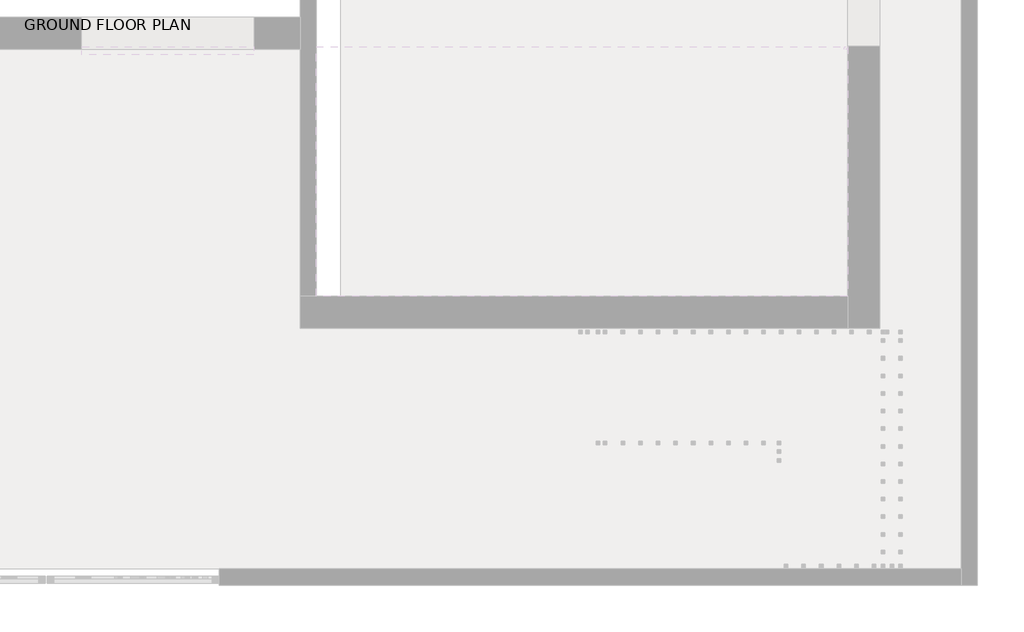
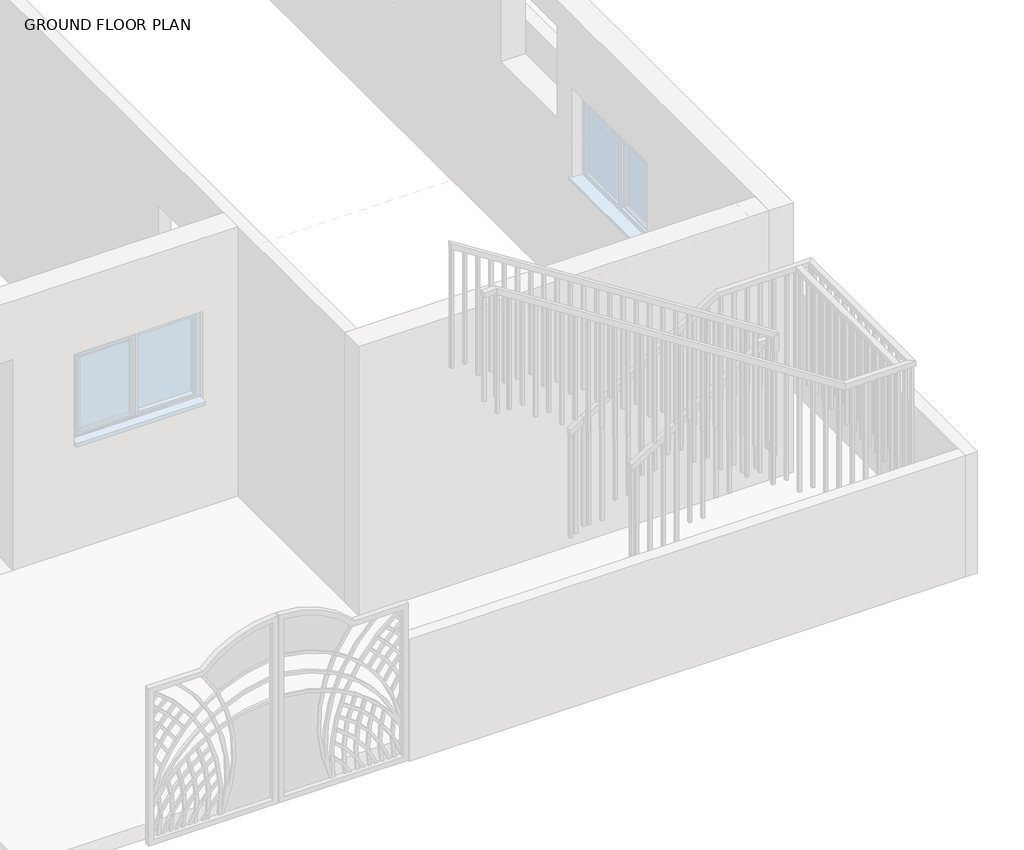
# One storey, part 11 of 23: 2 railings.
"""IFC4 building model written with IfcOpenShell, lengths in millimetres."""

from ifc_helpers import new_model, si_unit, frame, origin, place, context, project, spatial, polyline, outline, extrude, faceted_brep, element, save

model = new_model("IFC4")

# Units and contexts
model_context = context("Model", 3, world=origin())
ifc_project = project(units=[si_unit("LENGTHUNIT", "METRE", prefix="MILLI")], contexts=[model_context])

# Site, building, storey
site = spatial("IfcSite", under=ifc_project)
building = spatial("IfcBuilding", under=site)
storey = spatial("IfcBuildingStorey", under=building, Name="GROUND FLOOR PLAN", Elevation=487.68)

# Railings
placement = place(None, origin())
element("IfcRailing", 1, ObjectType="1100mm", at=placement, inside=storey, context=model_context, shape_type="SolidModel", body=[
    faceted_brep([(-8680.149573, -10220.0521308, 1912.8), (-8680.149573, -10220.0521308, 1853.4423995), (-8680.149573, -10270.0521308, 1853.4423995), (-8680.149573, -10270.0521308, 1912.8), (-7409.7306254, -10220.0521308, 2725.6), (-7395.1045513, -10220.0521308, 2675.6), (-7395.1045513, -10270.0521308, 2675.6), (-7409.7306254, -10270.0521308, 2725.6), (-6495.8132565, -10220.0521308, 2725.6), (-6495.8132565, -10220.0521308, 2675.6), (-6545.8132565, -10270.0521308, 2675.6), (-6545.8132565, -10270.0521308, 2725.6), (-6495.8132565, -11933.6860066, 2725.6), (-6495.8132565, -11933.6860066, 2675.6), (-6545.8132565, -11883.6860066, 2675.6), (-6545.8132565, -11883.6860066, 2725.6), (-7155.718398, -11933.6860066, 2725.6), (-7170.3479429, -11933.6860066, 2675.6), (-7170.3479429, -11883.6860066, 2675.6), (-7155.718398, -11883.6860066, 2725.6), (-10457.8773536, -11933.6860066, 4838.88), (-10457.8773536, -11883.6860066, 4838.88), (-10457.8773536, -11883.6860066, 4779.517542), (-10457.8773536, -11933.6860066, 4779.517542)], [[[0, 1, 2, 3]], [[1, 0, 4, 5]], [[2, 1, 5, 6]], [[3, 2, 6, 7]], [[0, 3, 7, 4]], [[5, 4, 8, 9]], [[6, 5, 9, 10]], [[7, 6, 10, 11]], [[4, 7, 11, 8]], [[9, 8, 12, 13]], [[10, 9, 13, 14]], [[11, 10, 14, 15]], [[8, 11, 15, 12]], [[13, 12, 16, 17]], [[14, 13, 17, 18]], [[15, 14, 18, 19]], [[12, 15, 19, 16]], [[20, 21, 22, 23]], [[17, 16, 20, 23]], [[18, 17, 23, 22]], [[19, 18, 22, 21]], [[16, 19, 21, 20]]]),
    extrude(outline(polyline([(4691.8007425, -10320.8132565), (4707.7999723, -10345.8132565), (3576.32, -10345.8132565), (3576.32, -10320.8132565), (4691.8007425, -10320.8132565)])), frame((0.0, -11921.1860066, 0.0), z_axis=(0.0, 1.0, 0.0), x_axis=(0.0, 0.0, 1.0)), (0.0, 0.0, 1.0), 25.0),
    extrude(outline(polyline([(4611.8045935, -10195.8132565), (4627.8038233, -10220.8132565), (3576.32, -10220.8132565), (3576.32, -10195.8132565), (4611.8045935, -10195.8132565)])), frame((0.0, -11921.1860066, 0.0), z_axis=(0.0, 1.0, 0.0), x_axis=(0.0, 0.0, 1.0)), (0.0, 0.0, 1.0), 25.0),
    extrude(outline(polyline([(4531.8084444, -10070.8132565), (4547.8076742, -10095.8132565), (3413.76, -10095.8132565), (3413.76, -10070.8132565), (4531.8084444, -10070.8132565)])), frame((0.0, -11921.1860066, 0.0), z_axis=(0.0, 1.0, 0.0), x_axis=(0.0, 0.0, 1.0)), (0.0, 0.0, 1.0), 25.0),
    extrude(outline(polyline([(4451.8122954, -9945.8132565), (4467.8115252, -9970.8132565), (3413.76, -9970.8132565), (3413.76, -9945.8132565), (4451.8122954, -9945.8132565)])), frame((0.0, -11921.1860066, 0.0), z_axis=(0.0, 1.0, 0.0), x_axis=(0.0, 0.0, 1.0)), (0.0, 0.0, 1.0), 25.0),
    extrude(outline(polyline([(4371.8161463, -9820.8132565), (4387.8153761, -9845.8132565), (3251.2, -9845.8132565), (3251.2, -9820.8132565), (4371.8161463, -9820.8132565)])), frame((0.0, -11921.1860066, 0.0), z_axis=(0.0, 1.0, 0.0), x_axis=(0.0, 0.0, 1.0)), (0.0, 0.0, 1.0), 25.0),
    extrude(outline(polyline([(4291.8423995, -9695.8132565), (4307.8371231, -9720.8132565), (3251.2, -9720.8132565), (3251.2, -9695.8132565), (4291.8423995, -9695.8132565)])), frame((0.0, -11921.1860066, 0.0), z_axis=(0.0, 1.0, 0.0), x_axis=(0.0, 0.0, 1.0)), (0.0, 0.0, 1.0), 25.0),
    extrude(outline(polyline([(4211.8238482, -9570.8132565), (4227.823078, -9595.8132565), (3088.64, -9595.8132565), (3088.64, -9570.8132565), (4211.8238482, -9570.8132565)])), frame((0.0, -11921.1860066, 0.0), z_axis=(0.0, 1.0, 0.0), x_axis=(0.0, 0.0, 1.0)), (0.0, 0.0, 1.0), 25.0),
    extrude(outline(polyline([(4131.8276992, -9445.8132565), (4147.826929, -9470.8132565), (3088.64, -9470.8132565), (3088.64, -9445.8132565), (4131.8276992, -9445.8132565)])), frame((0.0, -11921.1860066, 0.0), z_axis=(0.0, 1.0, 0.0), x_axis=(0.0, 0.0, 1.0)), (0.0, 0.0, 1.0), 25.0),
    extrude(outline(polyline([(4051.8315501, -9320.8132565), (4067.8307799, -9345.8132565), (2926.08, -9345.8132565), (2926.08, -9320.8132565), (4051.8315501, -9320.8132565)])), frame((0.0, -11921.1860066, 0.0), z_axis=(0.0, 1.0, 0.0), x_axis=(0.0, 0.0, 1.0)), (0.0, 0.0, 1.0), 25.0),
    extrude(outline(polyline([(3971.835401, -9195.8132565), (3987.8346309, -9220.8132565), (2926.08, -9220.8132565), (2926.08, -9195.8132565), (3971.835401, -9195.8132565)])), frame((0.0, -11921.1860066, 0.0), z_axis=(0.0, 1.0, 0.0), x_axis=(0.0, 0.0, 1.0)), (0.0, 0.0, 1.0), 25.0),
    extrude(outline(polyline([(3891.839252, -9070.8132565), (3907.8384818, -9095.8132565), (2763.52, -9095.8132565), (2763.52, -9070.8132565), (3891.839252, -9070.8132565)])), frame((0.0, -11921.1860066, 0.0), z_axis=(0.0, 1.0, 0.0), x_axis=(0.0, 0.0, 1.0)), (0.0, 0.0, 1.0), 25.0),
    extrude(outline(polyline([(3811.8431029, -8945.8132565), (3827.8423328, -8970.8132565), (2763.52, -8970.8132565), (2763.52, -8945.8132565), (3811.8431029, -8945.8132565)])), frame((0.0, -11921.1860066, 0.0), z_axis=(0.0, 1.0, 0.0), x_axis=(0.0, 0.0, 1.0)), (0.0, 0.0, 1.0), 25.0),
    extrude(outline(polyline([(3731.8469539, -8820.8132565), (3747.8461837, -8845.8132565), (2600.96, -8845.8132565), (2600.96, -8820.8132565), (3731.8469539, -8820.8132565)])), frame((0.0, -11921.1860066, 0.0), z_axis=(0.0, 1.0, 0.0), x_axis=(0.0, 0.0, 1.0)), (0.0, 0.0, 1.0), 25.0),
    extrude(outline(polyline([(3651.8508048, -8695.8132565), (3667.8500347, -8720.8132565), (2600.96, -8720.8132565), (2600.96, -8695.8132565), (3651.8508048, -8695.8132565)])), frame((0.0, -11921.1860066, 0.0), z_axis=(0.0, 1.0, 0.0), x_axis=(0.0, 0.0, 1.0)), (0.0, 0.0, 1.0), 25.0),
    extrude(outline(polyline([(3571.8546558, -8570.8132565), (3587.8538856, -8595.8132565), (2438.4, -8595.8132565), (2438.4, -8570.8132565), (3571.8546558, -8570.8132565)])), frame((0.0, -11921.1860066, 0.0), z_axis=(0.0, 1.0, 0.0), x_axis=(0.0, 0.0, 1.0)), (0.0, 0.0, 1.0), 25.0),
    extrude(outline(polyline([(3491.8585067, -8445.8132565), (3507.8577365, -8470.8132565), (2438.4, -8470.8132565), (2438.4, -8445.8132565), (3491.8585067, -8445.8132565)])), frame((0.0, -11921.1860066, 0.0), z_axis=(0.0, 1.0, 0.0), x_axis=(0.0, 0.0, 1.0)), (0.0, 0.0, 1.0), 25.0),
    extrude(outline(polyline([(3411.8623577, -8320.8132565), (3427.8615875, -8345.8132565), (2275.84, -8345.8132565), (2275.84, -8320.8132565), (3411.8623577, -8320.8132565)])), frame((0.0, -11921.1860066, 0.0), z_axis=(0.0, 1.0, 0.0), x_axis=(0.0, 0.0, 1.0)), (0.0, 0.0, 1.0), 25.0),
    extrude(outline(polyline([(3331.8662086, -8195.8132565), (3347.8654384, -8220.8132565), (2275.84, -8220.8132565), (2275.84, -8195.8132565), (3331.8662086, -8195.8132565)])), frame((0.0, -11921.1860066, 0.0), z_axis=(0.0, 1.0, 0.0), x_axis=(0.0, 0.0, 1.0)), (0.0, 0.0, 1.0), 25.0),
    extrude(outline(polyline([(3251.8700596, -8070.8132565), (3267.8692894, -8095.8132565), (2113.28, -8095.8132565), (2113.28, -8070.8132565), (3251.8700596, -8070.8132565)])), frame((0.0, -11921.1860066, 0.0), z_axis=(0.0, 1.0, 0.0), x_axis=(0.0, 0.0, 1.0)), (0.0, 0.0, 1.0), 25.0),
    extrude(outline(polyline([(3171.8739105, -7945.8132565), (3187.8731403, -7970.8132565), (2113.28, -7970.8132565), (2113.28, -7945.8132565), (3171.8739105, -7945.8132565)])), frame((0.0, -11921.1860066, 0.0), z_axis=(0.0, 1.0, 0.0), x_axis=(0.0, 0.0, 1.0)), (0.0, 0.0, 1.0), 25.0),
    extrude(outline(polyline([(3091.8777615, -7820.8132565), (3107.8769913, -7845.8132565), (1950.72, -7845.8132565), (1950.72, -7820.8132565), (3091.8777615, -7820.8132565)])), frame((0.0, -11921.1860066, 0.0), z_axis=(0.0, 1.0, 0.0), x_axis=(0.0, 0.0, 1.0)), (0.0, 0.0, 1.0), 25.0),
    extrude(outline(polyline([(3011.8816124, -7695.8132565), (3027.8808422, -7720.8132565), (1950.72, -7720.8132565), (1950.72, -7695.8132565), (3011.8816124, -7695.8132565)])), frame((0.0, -11921.1860066, 0.0), z_axis=(0.0, 1.0, 0.0), x_axis=(0.0, 0.0, 1.0)), (0.0, 0.0, 1.0), 25.0),
    extrude(outline(polyline([(2931.8854634, -7570.8132565), (2947.8846932, -7595.8132565), (1788.16, -7595.8132565), (1788.16, -7570.8132565), (2931.8854634, -7570.8132565)])), frame((0.0, -11921.1860066, 0.0), z_axis=(0.0, 1.0, 0.0), x_axis=(0.0, 0.0, 1.0)), (0.0, 0.0, 1.0), 25.0),
    extrude(outline(polyline([(2851.8893143, -7445.8132565), (2867.8885441, -7470.8132565), (1788.16, -7470.8132565), (1788.16, -7445.8132565), (2851.8893143, -7445.8132565)])), frame((0.0, -11921.1860066, 0.0), z_axis=(0.0, 1.0, 0.0), x_axis=(0.0, 0.0, 1.0)), (0.0, 0.0, 1.0), 25.0),
    extrude(outline(polyline([(2771.8931653, -7320.8132565), (2787.8923951, -7345.8132565), (1625.6, -7345.8132565), (1625.6, -7320.8132565), (2771.8931653, -7320.8132565)])), frame((0.0, -11921.1860066, 0.0), z_axis=(0.0, 1.0, 0.0), x_axis=(0.0, 0.0, 1.0)), (0.0, 0.0, 1.0), 25.0),
    extrude(outline(polyline([(2691.8970162, -7195.8132565), (2707.896246, -7220.8132565), (1625.6, -7220.8132565), (1625.6, -7195.8132565), (2691.8970162, -7195.8132565)])), frame((0.0, -11921.1860066, 0.0), z_axis=(0.0, 1.0, 0.0), x_axis=(0.0, 0.0, 1.0)), (0.0, 0.0, 1.0), 25.0),
    extrude(outline(polyline([(-7070.8132565, -11921.1860066), (-7095.8132565, -11921.1860066), (-7095.8132565, -11896.1860066), (-7070.8132565, -11896.1860066), (-7070.8132565, -11921.1860066)])), frame((0.0, 0.0, 1625.6), z_axis=(0.0, 0.0, 1.0), x_axis=(1.0, 0.0, 0.0)), (0.0, 0.0, 1.0), 1050.0),
    extrude(outline(polyline([(-6945.8132565, -11921.1860066), (-6970.8132565, -11921.1860066), (-6970.8132565, -11896.1860066), (-6945.8132565, -11896.1860066), (-6945.8132565, -11921.1860066)])), frame((0.0, 0.0, 1625.6), z_axis=(0.0, 0.0, 1.0), x_axis=(1.0, 0.0, 0.0)), (0.0, 0.0, 1.0), 1050.0),
    extrude(outline(polyline([(-6820.8132565, -11921.1860066), (-6845.8132565, -11921.1860066), (-6845.8132565, -11896.1860066), (-6820.8132565, -11896.1860066), (-6820.8132565, -11921.1860066)])), frame((0.0, 0.0, 1625.6), z_axis=(0.0, 0.0, 1.0), x_axis=(1.0, 0.0, 0.0)), (0.0, 0.0, 1.0), 1050.0),
    extrude(outline(polyline([(-6695.8132565, -11921.1860066), (-6720.8132565, -11921.1860066), (-6720.8132565, -11896.1860066), (-6695.8132565, -11896.1860066), (-6695.8132565, -11921.1860066)])), frame((0.0, 0.0, 1625.6), z_axis=(0.0, 0.0, 1.0), x_axis=(1.0, 0.0, 0.0)), (0.0, 0.0, 1.0), 1050.0),
    extrude(outline(polyline([(-6570.8132565, -11921.1860066), (-6595.8132565, -11921.1860066), (-6595.8132565, -11896.1860066), (-6570.8132565, -11896.1860066), (-6570.8132565, -11921.1860066)])), frame((0.0, 0.0, 1625.6), z_axis=(0.0, 0.0, 1.0), x_axis=(1.0, 0.0, 0.0)), (0.0, 0.0, 1.0), 1050.0),
    extrude(outline(polyline([(-6508.3132565, -11795.0521308), (-6508.3132565, -11820.0521308), (-6533.3132565, -11820.0521308), (-6533.3132565, -11795.0521308), (-6508.3132565, -11795.0521308)])), frame((0.0, 0.0, 1625.6), z_axis=(0.0, 0.0, 1.0), x_axis=(1.0, 0.0, 0.0)), (0.0, 0.0, 1.0), 1050.0),
    extrude(outline(polyline([(-6508.3132565, -11670.0521308), (-6508.3132565, -11695.0521308), (-6533.3132565, -11695.0521308), (-6533.3132565, -11670.0521308), (-6508.3132565, -11670.0521308)])), frame((0.0, 0.0, 1625.6), z_axis=(0.0, 0.0, 1.0), x_axis=(1.0, 0.0, 0.0)), (0.0, 0.0, 1.0), 1050.0),
    extrude(outline(polyline([(-6508.3132565, -11545.0521308), (-6508.3132565, -11570.0521308), (-6533.3132565, -11570.0521308), (-6533.3132565, -11545.0521308), (-6508.3132565, -11545.0521308)])), frame((0.0, 0.0, 1625.6), z_axis=(0.0, 0.0, 1.0), x_axis=(1.0, 0.0, 0.0)), (0.0, 0.0, 1.0), 1050.0),
    extrude(outline(polyline([(-6508.3132565, -11420.0521308), (-6508.3132565, -11445.0521308), (-6533.3132565, -11445.0521308), (-6533.3132565, -11420.0521308), (-6508.3132565, -11420.0521308)])), frame((0.0, 0.0, 1625.6), z_axis=(0.0, 0.0, 1.0), x_axis=(1.0, 0.0, 0.0)), (0.0, 0.0, 1.0), 1050.0),
    extrude(outline(polyline([(-6508.3132565, -11295.0521308), (-6508.3132565, -11320.0521308), (-6533.3132565, -11320.0521308), (-6533.3132565, -11295.0521308), (-6508.3132565, -11295.0521308)])), frame((0.0, 0.0, 1625.6), z_axis=(0.0, 0.0, 1.0), x_axis=(1.0, 0.0, 0.0)), (0.0, 0.0, 1.0), 1050.0),
    extrude(outline(polyline([(-6508.3132565, -11170.0521308), (-6508.3132565, -11195.0521308), (-6533.3132565, -11195.0521308), (-6533.3132565, -11170.0521308), (-6508.3132565, -11170.0521308)])), frame((0.0, 0.0, 1625.6), z_axis=(0.0, 0.0, 1.0), x_axis=(1.0, 0.0, 0.0)), (0.0, 0.0, 1.0), 1050.0),
    extrude(outline(polyline([(-6508.3132565, -11045.0521308), (-6508.3132565, -11070.0521308), (-6533.3132565, -11070.0521308), (-6533.3132565, -11045.0521308), (-6508.3132565, -11045.0521308)])), frame((0.0, 0.0, 1625.6), z_axis=(0.0, 0.0, 1.0), x_axis=(1.0, 0.0, 0.0)), (0.0, 0.0, 1.0), 1050.0),
    extrude(outline(polyline([(-6508.3132565, -10920.0521308), (-6508.3132565, -10945.0521308), (-6533.3132565, -10945.0521308), (-6533.3132565, -10920.0521308), (-6508.3132565, -10920.0521308)])), frame((0.0, 0.0, 1625.6), z_axis=(0.0, 0.0, 1.0), x_axis=(1.0, 0.0, 0.0)), (0.0, 0.0, 1.0), 1050.0),
    extrude(outline(polyline([(-6508.3132565, -10795.0521308), (-6508.3132565, -10820.0521308), (-6533.3132565, -10820.0521308), (-6533.3132565, -10795.0521308), (-6508.3132565, -10795.0521308)])), frame((0.0, 0.0, 1625.6), z_axis=(0.0, 0.0, 1.0), x_axis=(1.0, 0.0, 0.0)), (0.0, 0.0, 1.0), 1050.0),
    extrude(outline(polyline([(-6508.3132565, -10670.0521308), (-6508.3132565, -10695.0521308), (-6533.3132565, -10695.0521308), (-6533.3132565, -10670.0521308), (-6508.3132565, -10670.0521308)])), frame((0.0, 0.0, 1625.6), z_axis=(0.0, 0.0, 1.0), x_axis=(1.0, 0.0, 0.0)), (0.0, 0.0, 1.0), 1050.0),
    extrude(outline(polyline([(-6508.3132565, -10545.0521308), (-6508.3132565, -10570.0521308), (-6533.3132565, -10570.0521308), (-6533.3132565, -10545.0521308), (-6508.3132565, -10545.0521308)])), frame((0.0, 0.0, 1625.6), z_axis=(0.0, 0.0, 1.0), x_axis=(1.0, 0.0, 0.0)), (0.0, 0.0, 1.0), 1050.0),
    extrude(outline(polyline([(-6508.3132565, -10420.0521308), (-6508.3132565, -10445.0521308), (-6533.3132565, -10445.0521308), (-6533.3132565, -10420.0521308), (-6508.3132565, -10420.0521308)])), frame((0.0, 0.0, 1625.6), z_axis=(0.0, 0.0, 1.0), x_axis=(1.0, 0.0, 0.0)), (0.0, 0.0, 1.0), 1050.0),
    extrude(outline(polyline([(-6508.3132565, -10295.0521308), (-6508.3132565, -10320.0521308), (-6533.3132565, -10320.0521308), (-6533.3132565, -10295.0521308), (-6508.3132565, -10295.0521308)])), frame((0.0, 0.0, 1625.6), z_axis=(0.0, 0.0, 1.0), x_axis=(1.0, 0.0, 0.0)), (0.0, 0.0, 1.0), 1050.0),
    extrude(outline(polyline([(-6630.149573, -10232.5521308), (-6605.149573, -10232.5521308), (-6605.149573, -10257.5521308), (-6630.149573, -10257.5521308), (-6630.149573, -10232.5521308)])), frame((0.0, 0.0, 1625.6), z_axis=(0.0, 0.0, 1.0), x_axis=(1.0, 0.0, 0.0)), (0.0, 0.0, 1.0), 1050.0),
    extrude(outline(polyline([(-6755.149573, -10232.5521308), (-6730.149573, -10232.5521308), (-6730.149573, -10257.5521308), (-6755.149573, -10257.5521308), (-6755.149573, -10232.5521308)])), frame((0.0, 0.0, 1625.6), z_axis=(0.0, 0.0, 1.0), x_axis=(1.0, 0.0, 0.0)), (0.0, 0.0, 1.0), 1050.0),
    extrude(outline(polyline([(-6880.149573, -10232.5521308), (-6855.149573, -10232.5521308), (-6855.149573, -10257.5521308), (-6880.149573, -10257.5521308), (-6880.149573, -10232.5521308)])), frame((0.0, 0.0, 1625.6), z_axis=(0.0, 0.0, 1.0), x_axis=(1.0, 0.0, 0.0)), (0.0, 0.0, 1.0), 1050.0),
    extrude(outline(polyline([(-7005.149573, -10232.5521308), (-6980.149573, -10232.5521308), (-6980.149573, -10257.5521308), (-7005.149573, -10257.5521308), (-7005.149573, -10232.5521308)])), frame((0.0, 0.0, 1625.6), z_axis=(0.0, 0.0, 1.0), x_axis=(1.0, 0.0, 0.0)), (0.0, 0.0, 1.0), 1050.0),
    extrude(outline(polyline([(-7130.149573, -10232.5521308), (-7105.149573, -10232.5521308), (-7105.149573, -10257.5521308), (-7130.149573, -10257.5521308), (-7130.149573, -10232.5521308)])), frame((0.0, 0.0, 1625.6), z_axis=(0.0, 0.0, 1.0), x_axis=(1.0, 0.0, 0.0)), (0.0, 0.0, 1.0), 1050.0),
    extrude(outline(polyline([(-7255.149573, -10232.5521308), (-7230.149573, -10232.5521308), (-7230.149573, -10257.5521308), (-7255.149573, -10257.5521308), (-7255.149573, -10232.5521308)])), frame((0.0, 0.0, 1625.6), z_axis=(0.0, 0.0, 1.0), x_axis=(1.0, 0.0, 0.0)), (0.0, 0.0, 1.0), 1050.0),
    extrude(outline(polyline([(-7380.149573, -10232.5521308), (-7355.149573, -10232.5521308), (-7355.149573, -10257.5521308), (-7380.149573, -10257.5521308), (-7380.149573, -10232.5521308)])), frame((0.0, 0.0, 1625.6), z_axis=(0.0, 0.0, 1.0), x_axis=(1.0, 0.0, 0.0)), (0.0, 0.0, 1.0), 1050.0),
    extrude(outline(polyline([(1463.04, -7505.149573), (1463.04, -7480.149573), (2621.1891352, -7480.149573), (2605.1944115, -7505.149573), (1463.04, -7505.149573)])), frame((0.0, -10257.5521308, 0.0), z_axis=(0.0, 1.0, 0.0), x_axis=(0.0, 0.0, 1.0)), (0.0, 0.0, 1.0), 25.0),
    extrude(outline(polyline([(1463.04, -7630.149573), (1463.04, -7605.149573), (2541.2155169, -7605.149573), (2525.2207932, -7630.149573), (1463.04, -7630.149573)])), frame((0.0, -10257.5521308, 0.0), z_axis=(0.0, 1.0, 0.0), x_axis=(0.0, 0.0, 1.0)), (0.0, 0.0, 1.0), 25.0),
    extrude(outline(polyline([(1300.48, -7755.149573), (1300.48, -7730.149573), (2461.2418986, -7730.149573), (2445.2471749, -7755.149573), (1300.48, -7755.149573)])), frame((0.0, -10257.5521308, 0.0), z_axis=(0.0, 1.0, 0.0), x_axis=(0.0, 0.0, 1.0)), (0.0, 0.0, 1.0), 25.0),
    extrude(outline(polyline([(1300.48, -7880.149573), (1300.48, -7855.149573), (2381.2682803, -7855.149573), (2365.2735566, -7880.149573), (1300.48, -7880.149573)])), frame((0.0, -10257.5521308, 0.0), z_axis=(0.0, 1.0, 0.0), x_axis=(0.0, 0.0, 1.0)), (0.0, 0.0, 1.0), 25.0),
    extrude(outline(polyline([(1137.92, -8005.149573), (1137.92, -7980.149573), (2301.294662, -7980.149573), (2285.2999383, -8005.149573), (1137.92, -8005.149573)])), frame((0.0, -10257.5521308, 0.0), z_axis=(0.0, 1.0, 0.0), x_axis=(0.0, 0.0, 1.0)), (0.0, 0.0, 1.0), 25.0),
    extrude(outline(polyline([(1137.92, -8130.149573), (1137.92, -8105.149573), (2221.3210437, -8105.149573), (2205.32632, -8130.149573), (1137.92, -8130.149573)])), frame((0.0, -10257.5521308, 0.0), z_axis=(0.0, 1.0, 0.0), x_axis=(0.0, 0.0, 1.0)), (0.0, 0.0, 1.0), 25.0),
    extrude(outline(polyline([(975.36, -8255.149573), (975.36, -8230.149573), (2141.3474254, -8230.149573), (2125.3527017, -8255.149573), (975.36, -8255.149573)])), frame((0.0, -10257.5521308, 0.0), z_axis=(0.0, 1.0, 0.0), x_axis=(0.0, 0.0, 1.0)), (0.0, 0.0, 1.0), 25.0),
    extrude(outline(polyline([(975.36, -8380.149573), (975.36, -8355.149573), (2061.3738071, -8355.149573), (2045.3790834, -8380.149573), (975.36, -8380.149573)])), frame((0.0, -10257.5521308, 0.0), z_axis=(0.0, 1.0, 0.0), x_axis=(0.0, 0.0, 1.0)), (0.0, 0.0, 1.0), 25.0),
    extrude(outline(polyline([(812.8, -8505.149573), (812.8, -8480.149573), (1981.4001888, -8480.149573), (1965.4054651, -8505.149573), (812.8, -8505.149573)])), frame((0.0, -10257.5521308, 0.0), z_axis=(0.0, 1.0, 0.0), x_axis=(0.0, 0.0, 1.0)), (0.0, 0.0, 1.0), 25.0),
    extrude(outline(polyline([(812.8, -8630.149573), (812.8, -8605.149573), (1901.4265705, -8605.149573), (1885.4318468, -8630.149573), (812.8, -8630.149573)])), frame((0.0, -10257.5521308, 0.0), z_axis=(0.0, 1.0, 0.0), x_axis=(0.0, 0.0, 1.0)), (0.0, 0.0, 1.0), 25.0),
    extrude(outline(polyline([(-6508.3132565, -11896.1860066), (-6508.3132565, -11921.1860066), (-6533.3132565, -11921.1860066), (-6533.3132565, -11896.1860066), (-6508.3132565, -11896.1860066)])), frame((0.0, 0.0, 1625.6), z_axis=(0.0, 0.0, 1.0), x_axis=(1.0, 0.0, 0.0)), (0.0, 0.0, 1.0), 1050.0),
    extrude(outline(polyline([(-6533.3132565, -10232.5521308), (-6508.3132565, -10232.5521308), (-6508.3132565, -10257.5521308), (-6533.3132565, -10257.5521308), (-6533.3132565, -10232.5521308)])), frame((0.0, 0.0, 1625.6), z_axis=(0.0, 0.0, 1.0), x_axis=(1.0, 0.0, 0.0)), (0.0, 0.0, 1.0), 1050.0),
    extrude(outline(polyline([(4763.5183122, -10432.8773536), (4779.517542, -10457.8773536), (3576.32, -10457.8773536), (3576.32, -10432.8773536), (4763.5183122, -10432.8773536)])), frame((0.0, -11921.1860066, 0.0), z_axis=(0.0, 1.0, 0.0), x_axis=(0.0, 0.0, 1.0)), (0.0, 0.0, 1.0), 25.0),
    extrude(outline(polyline([(812.8, -8680.149573), (812.8, -8655.149573), (1869.4371231, -8655.149573), (1853.4423995, -8680.149573), (812.8, -8680.149573)])), frame((0.0, -10257.5521308, 0.0), z_axis=(0.0, 1.0, 0.0), x_axis=(0.0, 0.0, 1.0)), (0.0, 0.0, 1.0), 25.0),
])
element("IfcRailing", 2, ObjectType="1100mm", at=placement, inside=storey, context=model_context, shape_type="SolidModel", body=[
    faceted_brep([(-8805.870786, -10220.0521308, 1832.3649576), (-8805.870786, -10220.0521308, 1773.007357), (-8805.870786, -10270.0521308, 1773.007357), (-8805.870786, -10270.0521308, 1832.3649576), (-7409.7306254, -10220.0521308, 2725.6), (-7395.1045513, -10220.0521308, 2675.6), (-7395.1045513, -10270.0521308, 2675.6), (-7409.7306254, -10270.0521308, 2725.6), (-6621.5344696, -10220.0521308, 2725.6), (-6621.5344696, -10220.0521308, 2675.6), (-6671.5344696, -10270.0521308, 2675.6), (-6671.5344696, -10270.0521308, 2725.6), (-6621.5344696, -11933.6860066, 2725.6), (-6621.5344696, -11933.6860066, 2675.6), (-6671.5344696, -11883.6860066, 2675.6), (-6671.5344696, -11883.6860066, 2725.6), (-7155.718398, -11933.6860066, 2725.6), (-7170.3479429, -11933.6860066, 2675.6), (-7170.3479429, -11883.6860066, 2675.6), (-7155.718398, -11883.6860066, 2725.6), (-10457.8773536, -11933.6860066, 4838.88), (-10472.5068984, -11933.6860066, 4788.88), (-10472.5068984, -11883.6860066, 4788.88), (-10457.8773536, -11883.6860066, 4838.88), (-10583.5985666, -11933.6860066, 4838.88), (-10583.5985666, -11883.6860066, 4838.88), (-10583.5985666, -11883.6860066, 4788.88), (-10583.5985666, -11933.6860066, 4788.88)], [[[0, 1, 2, 3]], [[1, 0, 4, 5]], [[2, 1, 5, 6]], [[3, 2, 6, 7]], [[0, 3, 7, 4]], [[5, 4, 8, 9]], [[6, 5, 9, 10]], [[7, 6, 10, 11]], [[4, 7, 11, 8]], [[9, 8, 12, 13]], [[10, 9, 13, 14]], [[11, 10, 14, 15]], [[8, 11, 15, 12]], [[13, 12, 16, 17]], [[14, 13, 17, 18]], [[15, 14, 18, 19]], [[12, 15, 19, 16]], [[17, 16, 20, 21]], [[18, 17, 21, 22]], [[19, 18, 22, 23]], [[16, 19, 23, 20]], [[24, 25, 26, 27]], [[21, 20, 24, 27]], [[22, 21, 27, 26]], [[23, 22, 26, 25]], [[20, 23, 25, 24]]]),
    extrude(outline(polyline([(-10446.5344696, -11921.1860066), (-10471.5344696, -11921.1860066), (-10471.5344696, -11896.1860066), (-10446.5344696, -11896.1860066), (-10446.5344696, -11921.1860066)])), frame((0.0, 0.0, 3738.88), z_axis=(0.0, 0.0, 1.0), x_axis=(1.0, 0.0, 0.0)), (0.0, 0.0, 1.0), 1050.0),
    extrude(outline(polyline([(4692.2622966, -10321.5344696), (4708.2615264, -10346.5344696), (3576.32, -10346.5344696), (3576.32, -10321.5344696), (4692.2622966, -10321.5344696)])), frame((0.0, -11921.1860066, 0.0), z_axis=(0.0, 1.0, 0.0), x_axis=(0.0, 0.0, 1.0)), (0.0, 0.0, 1.0), 25.0),
    extrude(outline(polyline([(4612.2661476, -10196.5344696), (4628.2653774, -10221.5344696), (3576.32, -10221.5344696), (3576.32, -10196.5344696), (4612.2661476, -10196.5344696)])), frame((0.0, -11921.1860066, 0.0), z_axis=(0.0, 1.0, 0.0), x_axis=(0.0, 0.0, 1.0)), (0.0, 0.0, 1.0), 25.0),
    extrude(outline(polyline([(4532.2699985, -10071.5344696), (4548.2692283, -10096.5344696), (3413.76, -10096.5344696), (3413.76, -10071.5344696), (4532.2699985, -10071.5344696)])), frame((0.0, -11921.1860066, 0.0), z_axis=(0.0, 1.0, 0.0), x_axis=(0.0, 0.0, 1.0)), (0.0, 0.0, 1.0), 25.0),
    extrude(outline(polyline([(4452.2738495, -9946.5344696), (4468.2730793, -9971.5344696), (3413.76, -9971.5344696), (3413.76, -9946.5344696), (4452.2738495, -9946.5344696)])), frame((0.0, -11921.1860066, 0.0), z_axis=(0.0, 1.0, 0.0), x_axis=(0.0, 0.0, 1.0)), (0.0, 0.0, 1.0), 25.0),
    extrude(outline(polyline([(4372.2777004, -9821.5344696), (4388.2769302, -9846.5344696), (3251.2, -9846.5344696), (3251.2, -9821.5344696), (4372.2777004, -9821.5344696)])), frame((0.0, -11921.1860066, 0.0), z_axis=(0.0, 1.0, 0.0), x_axis=(0.0, 0.0, 1.0)), (0.0, 0.0, 1.0), 25.0),
    extrude(outline(polyline([(4292.2815514, -9696.5344696), (4308.2807812, -9721.5344696), (3251.2, -9721.5344696), (3251.2, -9696.5344696), (4292.2815514, -9696.5344696)])), frame((0.0, -11921.1860066, 0.0), z_axis=(0.0, 1.0, 0.0), x_axis=(0.0, 0.0, 1.0)), (0.0, 0.0, 1.0), 25.0),
    extrude(outline(polyline([(4212.2854023, -9571.5344696), (4228.2846321, -9596.5344696), (3088.64, -9596.5344696), (3088.64, -9571.5344696), (4212.2854023, -9571.5344696)])), frame((0.0, -11921.1860066, 0.0), z_axis=(0.0, 1.0, 0.0), x_axis=(0.0, 0.0, 1.0)), (0.0, 0.0, 1.0), 25.0),
    extrude(outline(polyline([(4132.2892533, -9446.5344696), (4148.2884831, -9471.5344696), (3088.64, -9471.5344696), (3088.64, -9446.5344696), (4132.2892533, -9446.5344696)])), frame((0.0, -11921.1860066, 0.0), z_axis=(0.0, 1.0, 0.0), x_axis=(0.0, 0.0, 1.0)), (0.0, 0.0, 1.0), 25.0),
    extrude(outline(polyline([(4052.2931042, -9321.5344696), (4068.292334, -9346.5344696), (2926.08, -9346.5344696), (2926.08, -9321.5344696), (4052.2931042, -9321.5344696)])), frame((0.0, -11921.1860066, 0.0), z_axis=(0.0, 1.0, 0.0), x_axis=(0.0, 0.0, 1.0)), (0.0, 0.0, 1.0), 25.0),
    extrude(outline(polyline([(3972.2969552, -9196.5344696), (3988.296185, -9221.5344696), (2926.08, -9221.5344696), (2926.08, -9196.5344696), (3972.2969552, -9196.5344696)])), frame((0.0, -11921.1860066, 0.0), z_axis=(0.0, 1.0, 0.0), x_axis=(0.0, 0.0, 1.0)), (0.0, 0.0, 1.0), 25.0),
    extrude(outline(polyline([(3892.3008061, -9071.5344696), (3908.3000359, -9096.5344696), (2763.52, -9096.5344696), (2763.52, -9071.5344696), (3892.3008061, -9071.5344696)])), frame((0.0, -11921.1860066, 0.0), z_axis=(0.0, 1.0, 0.0), x_axis=(0.0, 0.0, 1.0)), (0.0, 0.0, 1.0), 25.0),
    extrude(outline(polyline([(3812.3046571, -8946.5344696), (3828.3038869, -8971.5344696), (2763.52, -8971.5344696), (2763.52, -8946.5344696), (3812.3046571, -8946.5344696)])), frame((0.0, -11921.1860066, 0.0), z_axis=(0.0, 1.0, 0.0), x_axis=(0.0, 0.0, 1.0)), (0.0, 0.0, 1.0), 25.0),
    extrude(outline(polyline([(3732.308508, -8821.5344696), (3748.3077378, -8846.5344696), (2600.96, -8846.5344696), (2600.96, -8821.5344696), (3732.308508, -8821.5344696)])), frame((0.0, -11921.1860066, 0.0), z_axis=(0.0, 1.0, 0.0), x_axis=(0.0, 0.0, 1.0)), (0.0, 0.0, 1.0), 25.0),
    extrude(outline(polyline([(3652.312359, -8696.5344696), (3668.3115888, -8721.5344696), (2600.96, -8721.5344696), (2600.96, -8696.5344696), (3652.312359, -8696.5344696)])), frame((0.0, -11921.1860066, 0.0), z_axis=(0.0, 1.0, 0.0), x_axis=(0.0, 0.0, 1.0)), (0.0, 0.0, 1.0), 25.0),
    extrude(outline(polyline([(3572.3162099, -8571.5344696), (3588.3154397, -8596.5344696), (2438.4, -8596.5344696), (2438.4, -8571.5344696), (3572.3162099, -8571.5344696)])), frame((0.0, -11921.1860066, 0.0), z_axis=(0.0, 1.0, 0.0), x_axis=(0.0, 0.0, 1.0)), (0.0, 0.0, 1.0), 25.0),
    extrude(outline(polyline([(3492.3200609, -8446.5344696), (3508.3192907, -8471.5344696), (2438.4, -8471.5344696), (2438.4, -8446.5344696), (3492.3200609, -8446.5344696)])), frame((0.0, -11921.1860066, 0.0), z_axis=(0.0, 1.0, 0.0), x_axis=(0.0, 0.0, 1.0)), (0.0, 0.0, 1.0), 25.0),
    extrude(outline(polyline([(3412.3239118, -8321.5344696), (3428.3231416, -8346.5344696), (2275.84, -8346.5344696), (2275.84, -8321.5344696), (3412.3239118, -8321.5344696)])), frame((0.0, -11921.1860066, 0.0), z_axis=(0.0, 1.0, 0.0), x_axis=(0.0, 0.0, 1.0)), (0.0, 0.0, 1.0), 25.0),
    extrude(outline(polyline([(3332.3277628, -8196.5344696), (3348.3269926, -8221.5344696), (2275.84, -8221.5344696), (2275.84, -8196.5344696), (3332.3277628, -8196.5344696)])), frame((0.0, -11921.1860066, 0.0), z_axis=(0.0, 1.0, 0.0), x_axis=(0.0, 0.0, 1.0)), (0.0, 0.0, 1.0), 25.0),
    extrude(outline(polyline([(3252.3316137, -8071.5344696), (3268.3308435, -8096.5344696), (2113.28, -8096.5344696), (2113.28, -8071.5344696), (3252.3316137, -8071.5344696)])), frame((0.0, -11921.1860066, 0.0), z_axis=(0.0, 1.0, 0.0), x_axis=(0.0, 0.0, 1.0)), (0.0, 0.0, 1.0), 25.0),
    extrude(outline(polyline([(3172.3354647, -7946.5344696), (3188.3346945, -7971.5344696), (2113.28, -7971.5344696), (2113.28, -7946.5344696), (3172.3354647, -7946.5344696)])), frame((0.0, -11921.1860066, 0.0), z_axis=(0.0, 1.0, 0.0), x_axis=(0.0, 0.0, 1.0)), (0.0, 0.0, 1.0), 25.0),
    extrude(outline(polyline([(3092.4129874, -7821.5344696), (3108.4077111, -7846.5344696), (1950.72, -7846.5344696), (1950.72, -7821.5344696), (3092.4129874, -7821.5344696)])), frame((0.0, -11921.1860066, 0.0), z_axis=(0.0, 1.0, 0.0), x_axis=(0.0, 0.0, 1.0)), (0.0, 0.0, 1.0), 25.0),
    extrude(outline(polyline([(3012.4393691, -7696.5344696), (3028.4340928, -7721.5344696), (1950.72, -7721.5344696), (1950.72, -7696.5344696), (3012.4393691, -7696.5344696)])), frame((0.0, -11921.1860066, 0.0), z_axis=(0.0, 1.0, 0.0), x_axis=(0.0, 0.0, 1.0)), (0.0, 0.0, 1.0), 25.0),
    extrude(outline(polyline([(2932.4657508, -7571.5344696), (2948.4604745, -7596.5344696), (1788.16, -7596.5344696), (1788.16, -7571.5344696), (2932.4657508, -7571.5344696)])), frame((0.0, -11921.1860066, 0.0), z_axis=(0.0, 1.0, 0.0), x_axis=(0.0, 0.0, 1.0)), (0.0, 0.0, 1.0), 25.0),
    extrude(outline(polyline([(2852.4921325, -7446.5344696), (2868.4868562, -7471.5344696), (1788.16, -7471.5344696), (1788.16, -7446.5344696), (2852.4921325, -7446.5344696)])), frame((0.0, -11921.1860066, 0.0), z_axis=(0.0, 1.0, 0.0), x_axis=(0.0, 0.0, 1.0)), (0.0, 0.0, 1.0), 25.0),
    extrude(outline(polyline([(2772.3547194, -7321.5344696), (2788.3539492, -7346.5344696), (1625.6, -7346.5344696), (1625.6, -7321.5344696), (2772.3547194, -7321.5344696)])), frame((0.0, -11921.1860066, 0.0), z_axis=(0.0, 1.0, 0.0), x_axis=(0.0, 0.0, 1.0)), (0.0, 0.0, 1.0), 25.0),
    extrude(outline(polyline([(2692.3585703, -7196.5344696), (2708.3578001, -7221.5344696), (1625.6, -7221.5344696), (1625.6, -7196.5344696), (2692.3585703, -7196.5344696)])), frame((0.0, -11921.1860066, 0.0), z_axis=(0.0, 1.0, 0.0), x_axis=(0.0, 0.0, 1.0)), (0.0, 0.0, 1.0), 25.0),
    extrude(outline(polyline([(-7071.5344696, -11921.1860066), (-7096.5344696, -11921.1860066), (-7096.5344696, -11896.1860066), (-7071.5344696, -11896.1860066), (-7071.5344696, -11921.1860066)])), frame((0.0, 0.0, 1625.6), z_axis=(0.0, 0.0, 1.0), x_axis=(1.0, 0.0, 0.0)), (0.0, 0.0, 1.0), 1050.0),
    extrude(outline(polyline([(-6946.5344696, -11921.1860066), (-6971.5344696, -11921.1860066), (-6971.5344696, -11896.1860066), (-6946.5344696, -11896.1860066), (-6946.5344696, -11921.1860066)])), frame((0.0, 0.0, 1625.6), z_axis=(0.0, 0.0, 1.0), x_axis=(1.0, 0.0, 0.0)), (0.0, 0.0, 1.0), 1050.0),
    extrude(outline(polyline([(-6821.5344696, -11921.1860066), (-6846.5344696, -11921.1860066), (-6846.5344696, -11896.1860066), (-6821.5344696, -11896.1860066), (-6821.5344696, -11921.1860066)])), frame((0.0, 0.0, 1625.6), z_axis=(0.0, 0.0, 1.0), x_axis=(1.0, 0.0, 0.0)), (0.0, 0.0, 1.0), 1050.0),
    extrude(outline(polyline([(-6696.5344696, -11921.1860066), (-6721.5344696, -11921.1860066), (-6721.5344696, -11896.1860066), (-6696.5344696, -11896.1860066), (-6696.5344696, -11921.1860066)])), frame((0.0, 0.0, 1625.6), z_axis=(0.0, 0.0, 1.0), x_axis=(1.0, 0.0, 0.0)), (0.0, 0.0, 1.0), 1050.0),
    extrude(outline(polyline([(-6634.0344696, -11795.0521308), (-6634.0344696, -11820.0521308), (-6659.0344696, -11820.0521308), (-6659.0344696, -11795.0521308), (-6634.0344696, -11795.0521308)])), frame((0.0, 0.0, 1625.6), z_axis=(0.0, 0.0, 1.0), x_axis=(1.0, 0.0, 0.0)), (0.0, 0.0, 1.0), 1050.0),
    extrude(outline(polyline([(-6634.0344696, -11670.0521308), (-6634.0344696, -11695.0521308), (-6659.0344696, -11695.0521308), (-6659.0344696, -11670.0521308), (-6634.0344696, -11670.0521308)])), frame((0.0, 0.0, 1625.6), z_axis=(0.0, 0.0, 1.0), x_axis=(1.0, 0.0, 0.0)), (0.0, 0.0, 1.0), 1050.0),
    extrude(outline(polyline([(-6634.0344696, -11545.0521308), (-6634.0344696, -11570.0521308), (-6659.0344696, -11570.0521308), (-6659.0344696, -11545.0521308), (-6634.0344696, -11545.0521308)])), frame((0.0, 0.0, 1625.6), z_axis=(0.0, 0.0, 1.0), x_axis=(1.0, 0.0, 0.0)), (0.0, 0.0, 1.0), 1050.0),
    extrude(outline(polyline([(-6634.0344696, -11420.0521308), (-6634.0344696, -11445.0521308), (-6659.0344696, -11445.0521308), (-6659.0344696, -11420.0521308), (-6634.0344696, -11420.0521308)])), frame((0.0, 0.0, 1625.6), z_axis=(0.0, 0.0, 1.0), x_axis=(1.0, 0.0, 0.0)), (0.0, 0.0, 1.0), 1050.0),
    extrude(outline(polyline([(-6634.0344696, -11295.0521308), (-6634.0344696, -11320.0521308), (-6659.0344696, -11320.0521308), (-6659.0344696, -11295.0521308), (-6634.0344696, -11295.0521308)])), frame((0.0, 0.0, 1625.6), z_axis=(0.0, 0.0, 1.0), x_axis=(1.0, 0.0, 0.0)), (0.0, 0.0, 1.0), 1050.0),
    extrude(outline(polyline([(-6634.0344696, -11170.0521308), (-6634.0344696, -11195.0521308), (-6659.0344696, -11195.0521308), (-6659.0344696, -11170.0521308), (-6634.0344696, -11170.0521308)])), frame((0.0, 0.0, 1625.6), z_axis=(0.0, 0.0, 1.0), x_axis=(1.0, 0.0, 0.0)), (0.0, 0.0, 1.0), 1050.0),
    extrude(outline(polyline([(-6634.0344696, -11045.0521308), (-6634.0344696, -11070.0521308), (-6659.0344696, -11070.0521308), (-6659.0344696, -11045.0521308), (-6634.0344696, -11045.0521308)])), frame((0.0, 0.0, 1625.6), z_axis=(0.0, 0.0, 1.0), x_axis=(1.0, 0.0, 0.0)), (0.0, 0.0, 1.0), 1050.0),
    extrude(outline(polyline([(-6634.0344696, -10920.0521308), (-6634.0344696, -10945.0521308), (-6659.0344696, -10945.0521308), (-6659.0344696, -10920.0521308), (-6634.0344696, -10920.0521308)])), frame((0.0, 0.0, 1625.6), z_axis=(0.0, 0.0, 1.0), x_axis=(1.0, 0.0, 0.0)), (0.0, 0.0, 1.0), 1050.0),
    extrude(outline(polyline([(-6634.0344696, -10795.0521308), (-6634.0344696, -10820.0521308), (-6659.0344696, -10820.0521308), (-6659.0344696, -10795.0521308), (-6634.0344696, -10795.0521308)])), frame((0.0, 0.0, 1625.6), z_axis=(0.0, 0.0, 1.0), x_axis=(1.0, 0.0, 0.0)), (0.0, 0.0, 1.0), 1050.0),
    extrude(outline(polyline([(-6634.0344696, -10670.0521308), (-6634.0344696, -10695.0521308), (-6659.0344696, -10695.0521308), (-6659.0344696, -10670.0521308), (-6634.0344696, -10670.0521308)])), frame((0.0, 0.0, 1625.6), z_axis=(0.0, 0.0, 1.0), x_axis=(1.0, 0.0, 0.0)), (0.0, 0.0, 1.0), 1050.0),
    extrude(outline(polyline([(-6634.0344696, -10545.0521308), (-6634.0344696, -10570.0521308), (-6659.0344696, -10570.0521308), (-6659.0344696, -10545.0521308), (-6634.0344696, -10545.0521308)])), frame((0.0, 0.0, 1625.6), z_axis=(0.0, 0.0, 1.0), x_axis=(1.0, 0.0, 0.0)), (0.0, 0.0, 1.0), 1050.0),
    extrude(outline(polyline([(-6634.0344696, -10420.0521308), (-6634.0344696, -10445.0521308), (-6659.0344696, -10445.0521308), (-6659.0344696, -10420.0521308), (-6634.0344696, -10420.0521308)])), frame((0.0, 0.0, 1625.6), z_axis=(0.0, 0.0, 1.0), x_axis=(1.0, 0.0, 0.0)), (0.0, 0.0, 1.0), 1050.0),
    extrude(outline(polyline([(-6634.0344696, -10295.0521308), (-6634.0344696, -10320.0521308), (-6659.0344696, -10320.0521308), (-6659.0344696, -10295.0521308), (-6634.0344696, -10295.0521308)])), frame((0.0, 0.0, 1625.6), z_axis=(0.0, 0.0, 1.0), x_axis=(1.0, 0.0, 0.0)), (0.0, 0.0, 1.0), 1050.0),
    extrude(outline(polyline([(-6755.870786, -10232.5521308), (-6730.870786, -10232.5521308), (-6730.870786, -10257.5521308), (-6755.870786, -10257.5521308), (-6755.870786, -10232.5521308)])), frame((0.0, 0.0, 1625.6), z_axis=(0.0, 0.0, 1.0), x_axis=(1.0, 0.0, 0.0)), (0.0, 0.0, 1.0), 1050.0),
    extrude(outline(polyline([(-6880.870786, -10232.5521308), (-6855.870786, -10232.5521308), (-6855.870786, -10257.5521308), (-6880.870786, -10257.5521308), (-6880.870786, -10232.5521308)])), frame((0.0, 0.0, 1625.6), z_axis=(0.0, 0.0, 1.0), x_axis=(1.0, 0.0, 0.0)), (0.0, 0.0, 1.0), 1050.0),
    extrude(outline(polyline([(-7005.870786, -10232.5521308), (-6980.870786, -10232.5521308), (-6980.870786, -10257.5521308), (-7005.870786, -10257.5521308), (-7005.870786, -10232.5521308)])), frame((0.0, 0.0, 1625.6), z_axis=(0.0, 0.0, 1.0), x_axis=(1.0, 0.0, 0.0)), (0.0, 0.0, 1.0), 1050.0),
    extrude(outline(polyline([(-7130.870786, -10232.5521308), (-7105.870786, -10232.5521308), (-7105.870786, -10257.5521308), (-7130.870786, -10257.5521308), (-7130.870786, -10232.5521308)])), frame((0.0, 0.0, 1625.6), z_axis=(0.0, 0.0, 1.0), x_axis=(1.0, 0.0, 0.0)), (0.0, 0.0, 1.0), 1050.0),
    extrude(outline(polyline([(-7255.870786, -10232.5521308), (-7230.870786, -10232.5521308), (-7230.870786, -10257.5521308), (-7255.870786, -10257.5521308), (-7255.870786, -10232.5521308)])), frame((0.0, 0.0, 1625.6), z_axis=(0.0, 0.0, 1.0), x_axis=(1.0, 0.0, 0.0)), (0.0, 0.0, 1.0), 1050.0),
    extrude(outline(polyline([(-7380.870786, -10232.5521308), (-7355.870786, -10232.5521308), (-7355.870786, -10257.5521308), (-7380.870786, -10257.5521308), (-7380.870786, -10232.5521308)])), frame((0.0, 0.0, 1625.6), z_axis=(0.0, 0.0, 1.0), x_axis=(1.0, 0.0, 0.0)), (0.0, 0.0, 1.0), 1050.0),
    extrude(outline(polyline([(1463.04, -7505.870786), (1463.04, -7480.870786), (2620.7277111, -7480.870786), (2604.7329874, -7505.870786), (1463.04, -7505.870786)])), frame((0.0, -10257.5521308, 0.0), z_axis=(0.0, 1.0, 0.0), x_axis=(0.0, 0.0, 1.0)), (0.0, 0.0, 1.0), 25.0),
    extrude(outline(polyline([(1463.04, -7630.870786), (1463.04, -7605.870786), (2540.7540928, -7605.870786), (2524.7593691, -7630.870786), (1463.04, -7630.870786)])), frame((0.0, -10257.5521308, 0.0), z_axis=(0.0, 1.0, 0.0), x_axis=(0.0, 0.0, 1.0)), (0.0, 0.0, 1.0), 25.0),
    extrude(outline(polyline([(1300.48, -7755.870786), (1300.48, -7730.870786), (2460.7804745, -7730.870786), (2444.7857508, -7755.870786), (1300.48, -7755.870786)])), frame((0.0, -10257.5521308, 0.0), z_axis=(0.0, 1.0, 0.0), x_axis=(0.0, 0.0, 1.0)), (0.0, 0.0, 1.0), 25.0),
    extrude(outline(polyline([(1300.48, -7880.870786), (1300.48, -7855.870786), (2380.8068562, -7855.870786), (2364.8121325, -7880.870786), (1300.48, -7880.870786)])), frame((0.0, -10257.5521308, 0.0), z_axis=(0.0, 1.0, 0.0), x_axis=(0.0, 0.0, 1.0)), (0.0, 0.0, 1.0), 25.0),
    extrude(outline(polyline([(1137.92, -8005.870786), (1137.92, -7980.870786), (2300.8332379, -7980.870786), (2284.8385142, -8005.870786), (1137.92, -8005.870786)])), frame((0.0, -10257.5521308, 0.0), z_axis=(0.0, 1.0, 0.0), x_axis=(0.0, 0.0, 1.0)), (0.0, 0.0, 1.0), 25.0),
    extrude(outline(polyline([(1137.92, -8130.870786), (1137.92, -8105.870786), (2220.8596196, -8105.870786), (2204.8648959, -8130.870786), (1137.92, -8130.870786)])), frame((0.0, -10257.5521308, 0.0), z_axis=(0.0, 1.0, 0.0), x_axis=(0.0, 0.0, 1.0)), (0.0, 0.0, 1.0), 25.0),
    extrude(outline(polyline([(975.36, -8255.870786), (975.36, -8230.870786), (2140.8860012, -8230.870786), (2124.8912776, -8255.870786), (975.36, -8255.870786)])), frame((0.0, -10257.5521308, 0.0), z_axis=(0.0, 1.0, 0.0), x_axis=(0.0, 0.0, 1.0)), (0.0, 0.0, 1.0), 25.0),
    extrude(outline(polyline([(975.36, -8380.870786), (975.36, -8355.870786), (2060.9123829, -8355.870786), (2044.9176593, -8380.870786), (975.36, -8380.870786)])), frame((0.0, -10257.5521308, 0.0), z_axis=(0.0, 1.0, 0.0), x_axis=(0.0, 0.0, 1.0)), (0.0, 0.0, 1.0), 25.0),
    extrude(outline(polyline([(812.8, -8505.870786), (812.8, -8480.870786), (1980.9387646, -8480.870786), (1964.944041, -8505.870786), (812.8, -8505.870786)])), frame((0.0, -10257.5521308, 0.0), z_axis=(0.0, 1.0, 0.0), x_axis=(0.0, 0.0, 1.0)), (0.0, 0.0, 1.0), 25.0),
    extrude(outline(polyline([(812.8, -8630.870786), (812.8, -8605.870786), (1900.9651463, -8605.870786), (1884.9704227, -8630.870786), (812.8, -8630.870786)])), frame((0.0, -10257.5521308, 0.0), z_axis=(0.0, 1.0, 0.0), x_axis=(0.0, 0.0, 1.0)), (0.0, 0.0, 1.0), 25.0),
    extrude(outline(polyline([(772.3517667, -8755.870786), (772.3517667, -8730.870786), (1820.991528, -8730.870786), (1804.9968044, -8755.870786), (772.3517667, -8755.870786)])), frame((0.0, -10257.5521308, 0.0), z_axis=(0.0, 1.0, 0.0), x_axis=(0.0, 0.0, 1.0)), (0.0, 0.0, 1.0), 25.0),
    extrude(outline(polyline([(-6634.0344696, -11896.1860066), (-6634.0344696, -11921.1860066), (-6659.0344696, -11921.1860066), (-6659.0344696, -11896.1860066), (-6634.0344696, -11896.1860066)])), frame((0.0, 0.0, 1625.6), z_axis=(0.0, 0.0, 1.0), x_axis=(1.0, 0.0, 0.0)), (0.0, 0.0, 1.0), 1050.0),
    extrude(outline(polyline([(-6659.0344696, -10232.5521308), (-6634.0344696, -10232.5521308), (-6634.0344696, -10257.5521308), (-6659.0344696, -10257.5521308), (-6659.0344696, -10232.5521308)])), frame((0.0, 0.0, 1625.6), z_axis=(0.0, 0.0, 1.0), x_axis=(1.0, 0.0, 0.0)), (0.0, 0.0, 1.0), 1050.0),
    extrude(outline(polyline([(-10558.5985666, -11921.1860066), (-10583.5985666, -11921.1860066), (-10583.5985666, -11896.1860066), (-10558.5985666, -11896.1860066), (-10558.5985666, -11921.1860066)])), frame((0.0, 0.0, 3738.88), z_axis=(0.0, 0.0, 1.0), x_axis=(1.0, 0.0, 0.0)), (0.0, 0.0, 1.0), 1050.0),
    extrude(outline(polyline([(740.3623194, -8805.870786), (740.3623194, -8780.870786), (1789.0020807, -8780.870786), (1773.007357, -8805.870786), (740.3623194, -8805.870786)])), frame((0.0, -10257.5521308, 0.0), z_axis=(0.0, 1.0, 0.0), x_axis=(0.0, 0.0, 1.0)), (0.0, 0.0, 1.0), 25.0),
])

save(model, "model.ifc")

# Revit data of these elements
# Type "1100mm"
#   built-in parameter 1008612 = 0.019685 (stored number, unit not read)
#   built-in parameter 1008611 = 0.019685 (stored number, unit not read)
#   built-in parameter 1008609 = 0.902231 (stored number, unit not read)
#   built-in parameter 1008604 = 0.19685 (stored number, unit not read)
#   built-in parameter 1008603 = 0.164042 (stored number, unit not read)
#   Railing Height = 3.608924 ft
#   built-in parameter 1008630 = 2
#   built-in parameter 1008610 = 2
#   built-in parameter 1008608 = 1
#   built-in parameter 1008618 = Baluster_Square : 25mm
# Elements 1, 2 (IfcRailing, "1100mm")
#   Phase Created = New Construction
